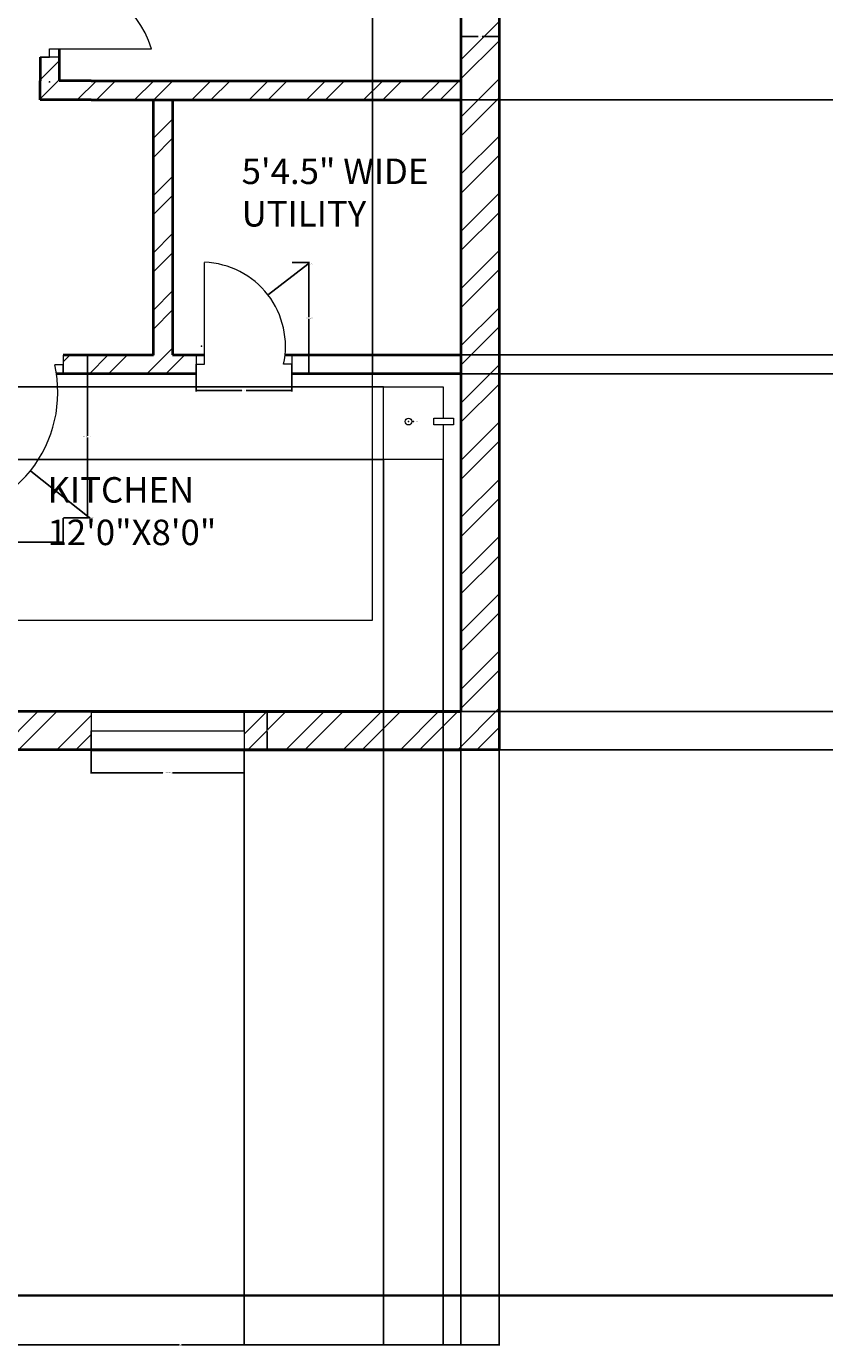
# Model space of a CAD drawing. Units: inches. Extents: x 1355 to 2746, y 1171 to 2751.
# Tile 3 of 24: x 1830 to 2017, y 1171 to 1482. Entities that reach past the tile are written whole.
import ezdxf

# ---------------------------------------------------------------- set-up
doc = ezdxf.new("R2010")
doc.units = ezdxf.units.IN
for name, color, linetype, lineweight in [('A-ANNO-DIMS', 2, 'Continuous', 18), ('A-ANNO-TTLB', 7, 'Continuous', 35), ('A-AREA-IDEN', 7, 'Continuous', 18), ('A-DOOR', 3, 'Continuous', 20), ('A-FLOR-CASE', 30, 'Continuous', 20), ('A-FLOR-FIXT', 9, 'Continuous', 18), ('A-GLAZ', 4, 'Continuous', 18), ('A-WALL', 7, 'Continuous', 40), ('A-WALL-PATT', 252, 'Continuous', 13)]:
    doc.layers.add(name, color=color, linetype=linetype, lineweight=lineweight)
doc.styles.get("Standard").update_dxf_attribs({"font": 'arial.ttf'})
doc.dimstyles.get("Standard").update_dxf_attribs({"dimtxt": 0.18, "dimasz": 0.18, "dimexe": 0.18, "dimexo": 0.0625, "dimgap": 0.09, "dimtad": 0, "dimtih": 1, "dimtoh": 1, "dimdec": 4, "dimzin": 0, "dimdsep": 46, "dimtxsty": 'Standard', "dimcen": 0.09, "dimadec": 0, "dimazin": 0, "dimtfac": 1, "dimtdec": 4, "dimtofl": 0, "dimtmove": 0, "dimatfit": 3, "dimfxl": 1, "dimtolj": 1, "dimtzin": 0, "dimarcsym": 0})

# ---------------------------------------------------------------- blocks, each defined once
blk = doc.blocks.new('WINDOW-PLAN-36')
for p, q in [((0, 9), (0, 0)), ((36, 4.5), (36, 9)), ((36, 9), (36, 0)), ((0, 0), (0, 4.5)), ((0, 4.5), (36, 4.5))]:
    blk.add_line(p, q)
blk = doc.blocks.new('DOOR-WC-SE')
for p, q in [((0, 21.41), (4.5, 21.41)), ((4.5, 21.41), (2.25, 21.41)), ((2.25, 21.41), (2.25, 19.41)), ((2.25, 0), (2.25, 2)), ((2.25, 2), (26.25, 2)), ((4.5, 0), (0, 0)), ((0, 0), (2.25, 0))]:
    blk.add_line(p, q)
blk.add_arc((2.25, -5.83), 25.25, 18.0786, 90)
blk = doc.blocks.new('DOOR-UTILITY-S')
for p, q in [((2, 2.25), (2, 26.25)), ((0, 4.5), (0, 0)), ((22.55, 4.5), (22.55, 0)), ((0, 0), (0, 2.25)), ((0, 2.25), (2, 2.25)), ((22.55, 2.25), (20.55, 2.25)), ((22.55, 0), (22.55, 2.25))]:
    blk.add_line(p, q)
blk.add_arc((1.26, 6.51), 19.76, 347.5613, 87.8563)
blk = doc.blocks.new('DOOR-KITCHEN-S')
for p, q in [((0, 38.25), (0, 33.75)), ((32.75, 38.25), (32.75, 33.89)), ((0, 33.75), (0, 36)), ((0, 36), (2, 36)), ((2, 36), (2, 0)), ((32.75, 36), (30.75, 36)), ((32.75, 33.89), (32.75, 36))]:
    blk.add_line(p, q)
blk.add_arc((2, 29.48), 29.48, 270, 12.7851)
blk = doc.blocks.new('*D43')
at = {"layer": 'A-ANNO-DIMS', "color": 0, "lineweight": -2, "transparency": 16777216}
for p, q in [((1844.71, 1311.24), (1844.71, 1305.72)), ((1880.71, 1311.24), (1880.71, 1305.72)), ((1844.89, 1305.9), (1861.59, 1305.9)), ((1880.53, 1305.9), (1863.83, 1305.9))]:
    blk.add_line(p, q, dxfattribs=at)
at = {"layer": 'A-ANNO-DIMS', "color": 0, "transparency": 16777216}
for points in [[(1844.89, 1305.93), (1844.89, 1305.87), (1844.71, 1305.9)], [(1880.53, 1305.93), (1880.53, 1305.87), (1880.71, 1305.9)]]:
    blk.add_solid(points, dxfattribs=at)
at = {"layer": 'Defpoints', "color": 0, "transparency": 16777216}
for p in [(1844.71, 1311.3), (1880.71, 1311.3), (1880.71, 1305.9)]:
    blk.add_point(p, dxfattribs=at)
at = {"layer": 'A-ANNO-DIMS', "color": 0, "transparency": 16777216, "insert": (1862.71, 1305.9), "char_height": 0.18, "attachment_point": 5}
blk.add_mtext('\\A1;WINDOW 36 TYP.', dxfattribs=at)
blk = doc.blocks.new('*D44')
at = {"layer": 'A-ANNO-DIMS', "color": 0, "lineweight": -2, "transparency": 16777216}
for p, q in [((1880.77, 1320.3), (1886.29, 1320.3)), ((1886.11, 1320.12), (1886.11, 1315.98)), ((1886.11, 1311.48), (1886.11, 1315.62)), ((1880.77, 1311.3), (1886.29, 1311.3))]:
    blk.add_line(p, q, dxfattribs=at)
at = {"layer": 'A-ANNO-DIMS', "color": 0, "transparency": 16777216}
for points in [[(1886.08, 1320.12), (1886.14, 1320.12), (1886.11, 1320.3)], [(1886.08, 1311.48), (1886.14, 1311.48), (1886.11, 1311.3)]]:
    blk.add_solid(points, dxfattribs=at)
at = {"layer": 'Defpoints', "color": 0, "transparency": 16777216}
for p in [(1880.71, 1320.3), (1886.11, 1320.3), (1880.71, 1311.3)]:
    blk.add_point(p, dxfattribs=at)
at = {"layer": 'A-ANNO-DIMS', "color": 0, "transparency": 16777216, "insert": (1886.11, 1315.8), "char_height": 0.18, "attachment_point": 5}
blk.add_mtext('\\A1;9 TYP.', dxfattribs=at)
blk = doc.blocks.new('*D52')
at = {"layer": 'A-ANNO-DIMS', "color": 0, "lineweight": -2, "transparency": 16777216}
for p, q in [((1931.71, 1482.72), (1931.71, 1479)), ((1940.71, 1482.72), (1940.71, 1479)), ((1931.89, 1479.18), (1935.75, 1479.18)), ((1940.53, 1479.18), (1936.67, 1479.18))]:
    blk.add_line(p, q, dxfattribs=at)
at = {"layer": 'A-ANNO-DIMS', "color": 0, "transparency": 16777216}
for points in [[(1931.89, 1479.21), (1931.89, 1479.15), (1931.71, 1479.18)], [(1940.53, 1479.21), (1940.53, 1479.15), (1940.71, 1479.18)]]:
    blk.add_solid(points, dxfattribs=at)
at = {"layer": 'Defpoints', "color": 0, "transparency": 16777216}
for p in [(1931.71, 1482.78), (1940.71, 1482.78), (1940.71, 1479.18)]:
    blk.add_point(p, dxfattribs=at)
at = {"layer": 'A-ANNO-DIMS', "color": 0, "transparency": 16777216, "insert": (1936.21, 1479.18), "char_height": 0.18, "attachment_point": 5}
blk.add_mtext('\\A1;9 TYP.', dxfattribs=at)
blk = doc.blocks.new('*D71')
at = {"layer": 'A-ANNO-DIMS', "color": 0, "lineweight": -2, "transparency": 16777216}
for p, q in [((1892.04, 1426.05), (1896.09, 1426.05)), ((1895.91, 1425.87), (1895.91, 1413.11)), ((1895.91, 1399.98), (1895.91, 1412.74)), ((1892.04, 1399.8), (1896.09, 1399.8))]:
    blk.add_line(p, q, dxfattribs=at)
at = {"layer": 'A-ANNO-DIMS', "color": 0, "transparency": 16777216}
for points in [[(1895.88, 1425.87), (1895.94, 1425.87), (1895.91, 1426.05)], [(1895.88, 1399.98), (1895.94, 1399.98), (1895.91, 1399.8)]]:
    blk.add_solid(points, dxfattribs=at)
at = {"layer": 'Defpoints', "color": 0, "transparency": 16777216}
for p in [(1891.97, 1426.05), (1895.91, 1426.05), (1891.97, 1399.8)]:
    blk.add_point(p, dxfattribs=at)
at = {"layer": 'A-ANNO-DIMS', "color": 0, "transparency": 16777216, "insert": (1895.91, 1412.93), "char_height": 0.18, "attachment_point": 5}
blk.add_mtext('\\A1;UTIL DOOR 26 TYP.', dxfattribs=at)
blk = doc.blocks.new('*D72')
at = {"layer": 'A-ANNO-DIMS', "color": 0, "lineweight": -2, "transparency": 16777216}
for p, q in [((1869.42, 1399.74), (1869.42, 1395.68)), ((1891.97, 1399.74), (1891.97, 1395.68)), ((1869.6, 1395.86), (1880.17, 1395.86)), ((1891.79, 1395.86), (1881.23, 1395.86))]:
    blk.add_line(p, q, dxfattribs=at)
at = {"layer": 'A-ANNO-DIMS', "color": 0, "transparency": 16777216}
for points in [[(1869.6, 1395.89), (1869.6, 1395.83), (1869.42, 1395.86)], [(1891.79, 1395.89), (1891.79, 1395.83), (1891.97, 1395.86)]]:
    blk.add_solid(points, dxfattribs=at)
at = {"layer": 'Defpoints', "color": 0, "transparency": 16777216}
for p in [(1869.42, 1399.8), (1891.97, 1399.8), (1891.97, 1395.86)]:
    blk.add_point(p, dxfattribs=at)
at = {"layer": 'A-ANNO-DIMS', "color": 0, "transparency": 16777216, "insert": (1880.7, 1395.86), "char_height": 0.18, "attachment_point": 5}
blk.add_mtext('\\A1;23 TYP.', dxfattribs=at)
blk = doc.blocks.new('*D73')
at = {"layer": 'A-ANNO-DIMS', "color": 0, "lineweight": -2, "transparency": 16777216}
for p, q in [((1838.22, 1404.17), (1844.07, 1404.17)), ((1843.89, 1403.99), (1843.89, 1385.22)), ((1843.89, 1366.1), (1843.89, 1384.86)), ((1838.22, 1365.92), (1844.07, 1365.92))]:
    blk.add_line(p, q, dxfattribs=at)
at = {"layer": 'A-ANNO-DIMS', "color": 0, "transparency": 16777216}
for points in [[(1843.86, 1403.99), (1843.92, 1403.99), (1843.89, 1404.17)], [(1843.86, 1366.1), (1843.92, 1366.1), (1843.89, 1365.92)]]:
    blk.add_solid(points, dxfattribs=at)
at = {"layer": 'Defpoints', "color": 0, "transparency": 16777216}
for p in [(1838.15, 1404.17), (1843.89, 1404.17), (1838.15, 1365.92)]:
    blk.add_point(p, dxfattribs=at)
at = {"layer": 'A-ANNO-DIMS', "color": 0, "transparency": 16777216, "insert": (1843.89, 1385.04), "char_height": 0.18, "attachment_point": 5}
blk.add_mtext('\\A1;KIT DOOR 38 TYP.', dxfattribs=at)
blk = doc.blocks.new('*D74')
at = {"layer": 'A-ANNO-DIMS', "color": 0, "lineweight": -2, "transparency": 16777216}
for p, q in [((1805.41, 1365.85), (1805.41, 1360)), ((1838.15, 1365.85), (1838.15, 1360)), ((1805.59, 1360.18), (1821.25, 1360.18)), ((1837.97, 1360.18), (1822.31, 1360.18))]:
    blk.add_line(p, q, dxfattribs=at)
at = {"layer": 'A-ANNO-DIMS', "color": 0, "transparency": 16777216}
for points in [[(1805.59, 1360.21), (1805.59, 1360.15), (1805.41, 1360.18)], [(1837.97, 1360.21), (1837.97, 1360.15), (1838.15, 1360.18)]]:
    blk.add_solid(points, dxfattribs=at)
at = {"layer": 'Defpoints', "color": 0, "transparency": 16777216}
for p in [(1805.41, 1365.92), (1838.15, 1365.92), (1838.15, 1360.18)]:
    blk.add_point(p, dxfattribs=at)
at = {"layer": 'A-ANNO-DIMS', "color": 0, "transparency": 16777216, "insert": (1821.78, 1360.18), "char_height": 0.18, "attachment_point": 5}
blk.add_mtext('\\A1;33 TYP.', dxfattribs=at)
blk = doc.blocks.new('*D106')
at = {"layer": 'A-ANNO-DIMS', "color": 0, "lineweight": -2, "transparency": 16777216}
for p, q in [((2031.09, 1557.85), (1407.53, 1557.85)), ((1407.71, 1557.67), (1407.71, 1434.76)), ((1407.71, 1311.48), (1407.71, 1434.39)), ((2080.33, 1311.3), (1407.53, 1311.3))]:
    blk.add_line(p, q, dxfattribs=at)
at = {"layer": 'A-ANNO-DIMS', "color": 0, "transparency": 16777216}
for points in [[(1407.68, 1557.67), (1407.74, 1557.67), (1407.71, 1557.85)], [(1407.68, 1311.48), (1407.74, 1311.48), (1407.71, 1311.3)]]:
    blk.add_solid(points, dxfattribs=at)
at = {"layer": 'Defpoints', "color": 0, "transparency": 16777216}
for p in [(1407.71, 1557.85), (2031.15, 1557.85), (2080.39, 1311.3)]:
    blk.add_point(p, dxfattribs=at)
at = {"layer": 'A-ANNO-DIMS', "color": 0, "transparency": 16777216, "insert": (1407.71, 1434.57), "char_height": 0.18, "attachment_point": 5}
blk.add_mtext('\\A1;246.54', dxfattribs=at)
blk = doc.blocks.new('*D141')
at = {"layer": 'A-ANNO-DIMS', "color": 0, "lineweight": -2, "transparency": 16777216}
for p, q in [((1799.71, 1320.24), (1799.71, 1171.06)), ((1931.71, 1320.24), (1931.71, 1171.06)), ((1799.89, 1171.24), (1865.43, 1171.24)), ((1931.53, 1171.24), (1865.99, 1171.24))]:
    blk.add_line(p, q, dxfattribs=at)
at = {"layer": 'A-ANNO-DIMS', "color": 0, "transparency": 16777216}
for points in [[(1799.89, 1171.27), (1799.89, 1171.21), (1799.71, 1171.24)], [(1931.53, 1171.27), (1931.53, 1171.21), (1931.71, 1171.24)]]:
    blk.add_solid(points, dxfattribs=at)
at = {"layer": 'Defpoints', "color": 0, "transparency": 16777216}
for p in [(1799.71, 1320.3), (1931.71, 1320.3), (1931.71, 1171.24)]:
    blk.add_point(p, dxfattribs=at)
at = {"layer": 'A-ANNO-DIMS', "color": 0, "transparency": 16777216, "insert": (1865.71, 1171.24), "char_height": 0.18, "attachment_point": 5}
blk.add_mtext('\\A1;132', dxfattribs=at)
blk = doc.blocks.new('*D142')
at = {"layer": 'A-ANNO-DIMS', "color": 0, "lineweight": -2, "transparency": 16777216}
for p, q in [((1931.77, 1399.8), (2648.07, 1399.8)), ((2647.89, 1399.62), (2647.89, 1360.23)), ((2647.89, 1320.48), (2647.89, 1359.87)), ((1931.77, 1320.3), (2648.07, 1320.3))]:
    blk.add_line(p, q, dxfattribs=at)
at = {"layer": 'A-ANNO-DIMS', "color": 0, "transparency": 16777216}
for points in [[(2647.86, 1399.62), (2647.92, 1399.62), (2647.89, 1399.8)], [(2647.86, 1320.48), (2647.92, 1320.48), (2647.89, 1320.3)]]:
    blk.add_solid(points, dxfattribs=at)
at = {"layer": 'Defpoints', "color": 0, "transparency": 16777216}
for p in [(1931.71, 1399.8), (2647.89, 1399.8), (1931.71, 1320.3)]:
    blk.add_point(p, dxfattribs=at)
at = {"layer": 'A-ANNO-DIMS', "color": 0, "transparency": 16777216, "insert": (2647.89, 1360.05), "char_height": 0.18, "attachment_point": 5}
blk.add_mtext('\\A1;79.5', dxfattribs=at)
blk = doc.blocks.new('*D143')
at = {"layer": 'A-ANNO-DIMS', "color": 0, "lineweight": -2, "transparency": 16777216}
for p, q in [((1931.77, 1464.3), (2648.07, 1464.3)), ((2647.89, 1464.12), (2647.89, 1434.48)), ((2647.89, 1404.48), (2647.89, 1434.12)), ((1931.77, 1404.3), (2648.07, 1404.3))]:
    blk.add_line(p, q, dxfattribs=at)
at = {"layer": 'A-ANNO-DIMS', "color": 0, "transparency": 16777216}
for points in [[(2647.86, 1464.12), (2647.92, 1464.12), (2647.89, 1464.3)], [(2647.86, 1404.48), (2647.92, 1404.48), (2647.89, 1404.3)]]:
    blk.add_solid(points, dxfattribs=at)
at = {"layer": 'Defpoints', "color": 0, "transparency": 16777216}
for p in [(1931.71, 1464.3), (2647.89, 1464.3), (1931.71, 1404.3)]:
    blk.add_point(p, dxfattribs=at)
at = {"layer": 'A-ANNO-DIMS', "color": 0, "transparency": 16777216, "insert": (2647.89, 1434.3), "char_height": 0.18, "attachment_point": 5}
blk.add_mtext('\\A1;60', dxfattribs=at)
blk = doc.blocks.new('*D144')
at = {"layer": 'A-ANNO-DIMS', "color": 0, "lineweight": -2, "transparency": 16777216}
for p, q in [((1880.71, 1311.24), (1880.71, 1171.06)), ((1940.71, 1311.24), (1940.71, 1171.06)), ((1880.89, 1171.24), (1910.49, 1171.24)), ((1940.53, 1171.24), (1910.93, 1171.24))]:
    blk.add_line(p, q, dxfattribs=at)
at = {"layer": 'A-ANNO-DIMS', "color": 0, "transparency": 16777216}
for points in [[(1880.89, 1171.27), (1880.89, 1171.21), (1880.71, 1171.24)], [(1940.53, 1171.27), (1940.53, 1171.21), (1940.71, 1171.24)]]:
    blk.add_solid(points, dxfattribs=at)
at = {"layer": 'Defpoints', "color": 0, "transparency": 16777216}
for p in [(1880.71, 1311.3), (1940.71, 1311.3), (1940.71, 1171.24)]:
    blk.add_point(p, dxfattribs=at)
at = {"layer": 'A-ANNO-DIMS', "color": 0, "transparency": 16777216, "insert": (1910.71, 1171.24), "char_height": 0.18, "attachment_point": 5}
blk.add_mtext('\\A1;60', dxfattribs=at)
blk = doc.blocks.new('*D145')
at = {"layer": 'A-ANNO-DIMS', "color": 0, "lineweight": -2, "transparency": 16777216}
for p, q in [((1910.88, 1399.86), (1910.88, 2716.58)), ((1911.06, 2716.4), (1920.83, 2716.4)), ((1931.53, 2716.4), (1921.76, 2716.4)), ((1931.71, 1399.86), (1931.71, 2716.58))]:
    blk.add_line(p, q, dxfattribs=at)
at = {"layer": 'A-ANNO-DIMS', "color": 0, "transparency": 16777216}
for points in [[(1911.06, 2716.43), (1911.06, 2716.37), (1910.88, 2716.4)], [(1931.53, 2716.43), (1931.53, 2716.37), (1931.71, 2716.4)]]:
    blk.add_solid(points, dxfattribs=at)
at = {"layer": 'Defpoints', "color": 0, "transparency": 16777216}
for p in [(1931.71, 2716.4), (1910.88, 1399.8), (1931.71, 1399.8)]:
    blk.add_point(p, dxfattribs=at)
at = {"layer": 'A-ANNO-DIMS', "color": 0, "transparency": 16777216, "insert": (1921.3, 2716.4), "char_height": 0.18, "attachment_point": 5}
blk.add_mtext('\\A1;20.824', dxfattribs=at)
blk = doc.blocks.new('*D146')
at = {"layer": 'A-ANNO-DIMS', "color": 0, "lineweight": -2, "transparency": 16777216}
for p, q in [((1913.53, 1379.56), (1913.53, 1171.06)), ((1927.55, 1379.56), (1927.55, 1171.06)), ((1913.71, 1171.24), (1920.08, 1171.24)), ((1927.37, 1171.24), (1920.99, 1171.24))]:
    blk.add_line(p, q, dxfattribs=at)
at = {"layer": 'A-ANNO-DIMS', "color": 0, "transparency": 16777216}
for points in [[(1913.71, 1171.27), (1913.71, 1171.21), (1913.53, 1171.24)], [(1927.37, 1171.27), (1927.37, 1171.21), (1927.55, 1171.24)]]:
    blk.add_solid(points, dxfattribs=at)
at = {"layer": 'Defpoints', "color": 0, "transparency": 16777216}
for p in [(1913.53, 1379.62), (1927.55, 1379.62), (1927.55, 1171.24)]:
    blk.add_point(p, dxfattribs=at)
at = {"layer": 'A-ANNO-DIMS', "color": 0, "transparency": 16777216, "insert": (1920.54, 1171.24), "char_height": 0.18, "attachment_point": 5}
blk.add_mtext('\\A1;14.014', dxfattribs=at)
blk = doc.blocks.new('*D147')
at = {"layer": 'A-ANNO-DIMS', "color": 0, "lineweight": -2, "transparency": 16777216}
for p, q in [((1913.47, 1396.75), (1407.53, 1396.75)), ((1407.71, 1396.57), (1407.71, 1388.37)), ((1407.71, 1379.8), (1407.71, 1388.01)), ((1913.47, 1379.62), (1407.53, 1379.62))]:
    blk.add_line(p, q, dxfattribs=at)
at = {"layer": 'A-ANNO-DIMS', "color": 0, "transparency": 16777216}
for points in [[(1407.68, 1396.57), (1407.74, 1396.57), (1407.71, 1396.75)], [(1407.68, 1379.8), (1407.74, 1379.8), (1407.71, 1379.62)]]:
    blk.add_solid(points, dxfattribs=at)
at = {"layer": 'Defpoints', "color": 0, "transparency": 16777216}
for p in [(1407.71, 1396.75), (1913.53, 1396.75), (1913.53, 1379.62)]:
    blk.add_point(p, dxfattribs=at)
at = {"layer": 'A-ANNO-DIMS', "color": 0, "transparency": 16777216, "insert": (1407.71, 1388.19), "char_height": 0.18, "attachment_point": 5}
blk.add_mtext('\\A1;17.13', dxfattribs=at)
blk = doc.blocks.new('*D149')
at = {"layer": 'A-ANNO-DIMS', "color": 0, "lineweight": -2, "transparency": 16777216}
for p, q in [((1919.3, 1388.57), (1919.48, 1388.57)), ((1919.39, 1388.48), (1919.39, 1388.66)), ((1920.65, 1388.57), (1920.36, 1388.57))]:
    blk.add_line(p, q, dxfattribs=at)
at = {"layer": 'A-ANNO-DIMS', "color": 0, "transparency": 16777216}
blk.add_solid([(1920.36, 1388.6), (1920.36, 1388.54), (1920.18, 1388.57)], dxfattribs=at)
at = {"layer": 'Defpoints', "color": 0, "transparency": 16777216}
for p in [(1918.6, 1388.56), (1920.18, 1388.57)]:
    blk.add_point(p, dxfattribs=at)
at = {"layer": 'A-ANNO-DIMS', "color": 0, "transparency": 16777216, "insert": (1921.08, 1388.57), "char_height": 0.18, "attachment_point": 5}
blk.add_mtext('\\A1;∅1.58', dxfattribs=at)
blk = doc.blocks.new('*D151')
at = {"layer": 'A-ANNO-DIMS', "color": 0, "lineweight": -2, "transparency": 16777216}
for p, q in [((1807.32, 1395.39), (1807.5, 1395.39)), ((1807.41, 1395.3), (1807.41, 1395.48)), ((1844.26, 1365.96), (1830.58, 1376.89)), ((1844.44, 1365.96), (1844.26, 1365.96))]:
    blk.add_line(p, q, dxfattribs=at)
at = {"layer": 'A-ANNO-DIMS', "color": 0, "transparency": 16777216}
blk.add_solid([(1830.6, 1376.91), (1830.56, 1376.86), (1830.44, 1377)], dxfattribs=at)
at = {"layer": 'Defpoints', "color": 0, "transparency": 16777216}
for p in [(1807.41, 1395.39), (1830.44, 1377)]:
    blk.add_point(p, dxfattribs=at)
at = {"layer": 'A-ANNO-DIMS', "color": 0, "transparency": 16777216, "insert": (1844.99, 1365.96), "char_height": 0.18, "attachment_point": 5}
blk.add_mtext('\\A1;R29.477', dxfattribs=at)
blk = doc.blocks.new('*D161')
at = {"layer": 'A-ANNO-DIMS', "color": 0, "lineweight": -2, "transparency": 16777216}
for p, q in [((1858.68, 1501.2), (1849.89, 1489.09)), ((1858.86, 1501.2), (1858.68, 1501.2)), ((1834.87, 1468.51), (1835.05, 1468.51)), ((1834.96, 1468.42), (1834.96, 1468.6))]:
    blk.add_line(p, q, dxfattribs=at)
at = {"layer": 'A-ANNO-DIMS', "color": 0, "transparency": 16777216}
blk.add_solid([(1849.87, 1489.1), (1849.91, 1489.07), (1849.78, 1488.94)], dxfattribs=at)
at = {"layer": 'Defpoints', "color": 0, "transparency": 16777216}
for p in [(1849.78, 1488.94), (1834.96, 1468.51)]:
    blk.add_point(p, dxfattribs=at)
at = {"layer": 'A-ANNO-DIMS', "color": 0, "transparency": 16777216, "insert": (1859.41, 1501.2), "char_height": 0.18, "attachment_point": 5}
blk.add_mtext('\\A1;R25.246', dxfattribs=at)
blk = doc.blocks.new('*D163')
at = {"layer": 'A-ANNO-DIMS', "color": 0, "lineweight": -2, "transparency": 16777216}
for p, q in [((1895.69, 1425.64), (1886.45, 1418.5)), ((1895.87, 1425.64), (1895.69, 1425.64)), ((1870.59, 1406.31), (1870.77, 1406.31)), ((1870.68, 1406.22), (1870.68, 1406.4))]:
    blk.add_line(p, q, dxfattribs=at)
at = {"layer": 'A-ANNO-DIMS', "color": 0, "transparency": 16777216}
blk.add_solid([(1886.43, 1418.53), (1886.47, 1418.48), (1886.31, 1418.39)], dxfattribs=at)
at = {"layer": 'Defpoints', "color": 0, "transparency": 16777216}
for p in [(1886.31, 1418.39), (1870.68, 1406.31)]:
    blk.add_point(p, dxfattribs=at)
at = {"layer": 'A-ANNO-DIMS', "color": 0, "transparency": 16777216, "insert": (1896.35, 1425.64), "char_height": 0.18, "attachment_point": 5}
blk.add_mtext('\\A1;R19.76', dxfattribs=at)

msp = doc.modelspace()

# ---------------------------------------------------------------- hatches: boundary and pattern name
at = {"layer": 'A-WALL-PATT'}
h = msp.add_hatch(dxfattribs=at)
h.set_pattern_fill('ANSI32', color=256)
h.paths.add_polyline_path([(1660.2083, 2139.3018), (1614.5977, 2139.3018), (1614.5977, 2130.3018), (1655.7083, 2130.3018), (1655.7083, 1981.8018), (1660.2083, 1981.8018), (1660.2083, 2090.7225), (1692.5832, 2090.7225), (1692.5832, 2095.2225), (1660.2083, 2095.2225)])
h.paths.add_polyline_path([(1523.7083, 2130.3018), (1554.5977, 2130.3018), (1554.5977, 2134.8018), (1554.5977, 2139.3018), (1514.7083, 2139.3018), (1514.7083, 2071.8385), (1523.7083, 2071.8385)])
h.paths.add_polyline_path([(1940.7083, 2139.3018), (1883.7928, 2139.3018), (1883.7928, 2130.3018), (1931.7083, 2130.3018), (1931.7083, 2098.3333), (1940.7083, 2098.3333)])
h.paths.add_polyline_path([(1799.7083, 2130.3018), (1823.7928, 2130.3018), (1823.7928, 2134.8018), (1823.7928, 2139.3018), (1795.2083, 2139.3018), (1795.2083, 2130.3018), (1795.2083, 2095.2225), (1759.2134, 2095.2225), (1759.2134, 2090.7225), (1795.2083, 2090.7225), (1795.2083, 1981.8018), (1799.7083, 1981.8018), (1799.7083, 1986.3018)])
h.paths.add_polyline_path([(1940.7083, 2038.3333), (1931.7083, 2038.3333), (1931.7083, 1986.3018), (1832.7083, 1986.3018), (1832.7083, 1947.1338), (1837.2083, 1947.1338), (1837.2083, 1981.8018), (1931.7083, 1981.8018), (1931.7083, 1967.1939), (1940.7083, 1967.1939)])
h.paths.add_polyline_path([(1940.7083, 1943.1939), (1931.7083, 1943.1939), (1931.7083, 1921.8018), (1837.2083, 1921.8018), (1837.2083, 1926.0511), (1832.7083, 1926.0511), (1832.7083, 1917.3018), (1931.7083, 1917.3018), (1931.7083, 1908.3321), (1940.7083, 1908.3321)])
h.paths.add_polyline_path([(1940.7083, 1884.3321), (1931.7083, 1884.3321), (1931.7083, 1869.3018), (1899.4583, 1869.3018), (1899.4583, 1864.8018), (1931.7083, 1864.8018), (1931.7083, 1773.3018), (1786.5143, 1773.3018), (1786.5143, 1764.3018), (1844.7083, 1764.3018), (1844.7083, 1748.9343), (1853.7083, 1748.9343), (1853.7083, 1764.3018), (1931.7083, 1764.3018), (1931.7083, 1652.9424), (1940.7083, 1652.9424)])
h.paths.add_polyline_path([(1799.7083, 1864.8018), (1806.0522, 1864.8018), (1806.0522, 1867.0518), (1806.0522, 1869.3018), (1799.7083, 1869.3018), (1799.7083, 1917.3018), (1799.7083, 1921.8018), (1795.2083, 1921.8018), (1795.2083, 1773.3018), (1799.7083, 1773.3018)])
h.paths.add_polyline_path([(1872.8988, 1867.0518), (1872.8988, 1869.3018), (1867.2083, 1869.3018), (1867.2083, 1917.3018), (1862.7083, 1917.3018), (1862.7083, 1869.3018), (1836.9546, 1869.3018), (1836.9546, 1864.8018), (1862.7083, 1864.8018), (1872.8988, 1864.8018)])
h.paths.add_polyline_path([(1749.2197, 1773.3018), (1655.7083, 1773.3018), (1523.7083, 1773.3018), (1523.7083, 1828.4963), (1514.7083, 1828.4963), (1514.7083, 1753.9033), (1519.2083, 1753.9033), (1523.7083, 1753.9033), (1523.7083, 1764.3018), (1655.7083, 1764.3018), (1749.2197, 1764.3018), (1749.2197, 1768.8018)])
h.paths.add_polyline_path([(1660.2083, 1921.8018), (1655.7083, 1921.8018), (1655.7083, 1917.3018), (1655.7083, 1773.3018), (1660.2083, 1773.3018)])
h.paths.add_polyline_path([(1523.7083, 2011.8385), (1514.7083, 2011.8385), (1514.7083, 1973.114), (1519.2083, 1973.114), (1523.7083, 1973.114), (1523.7083, 1976.8227), (1523.7083, 1981.8018), (1618.2083, 1981.8018), (1618.2083, 1921.8018), (1553.707, 1921.8018), (1553.707, 1917.3018), (1622.7083, 1917.3018), (1622.7083, 1919.5518), (1622.7083, 1921.8018), (1622.7083, 1986.3018), (1523.7083, 1986.3018)])
h.paths.add_polyline_path([(1529.6686, 1919.5518), (1529.6686, 1921.8018), (1523.7083, 1921.8018), (1523.7083, 1949.114), (1514.7083, 1949.114), (1514.7083, 1888.4963), (1523.7083, 1888.4963), (1523.7083, 1917.3018), (1529.6686, 1917.3018)])
h.paths.add_polyline_path([(1538.9419, 1775.643), (1585.5504, 1775.643), (1585.5504, 1798.0318), (1538.9419, 1798.0318)], flags=25)
h.paths.add_polyline_path([(1696.7097, 1497.3356), (1769.5651, 1497.3356), (1769.5651, 1523.4559), (1696.7097, 1523.4559)], flags=9)
h.paths.add_polyline_path([(1629.1643, 1230.5133), (1877.0879, 1230.5133), (1877.0879, 1267.606), (1629.1643, 1267.606)], flags=9)
h.paths.add_polyline_path([(2533.4462, 2215.4033), (2579.9292, 2215.4033), (2579.9292, 2231.889), (2533.4462, 2231.889)], flags=9)
h.paths.add_polyline_path([(2540.822, 2515.6945), (2594.2245, 2515.6945), (2594.2245, 2545.5463), (2540.822, 2545.5463)], flags=9)
h.paths.add_polyline_path([(2535.9857, 2588.2819), (2582.4687, 2588.2819), (2582.4687, 2604.7675), (2535.9857, 2604.7675)], flags=9)
h.paths.add_polyline_path([(2537.1627, 2617.1172), (2649.1245, 2617.1172), (2649.1245, 2633.6029), (2537.1627, 2633.6029)], flags=9)
h.paths.add_polyline_path([(2218.0051, 2168.228), (2363.9573, 2168.228), (2363.9573, 2205.3208), (2218.0051, 2205.3208)], flags=9)
h.paths.add_polyline_path([(1650.2156, 2165.3631), (1800.3547, 2165.3631), (1800.3547, 2202.4559), (1650.2156, 2202.4559)], flags=9)
h.paths.add_polyline_path([(2553.9592, 1610.7663), (2588.4203, 1610.7663), (2588.4203, 1660.2233), (2553.9592, 1660.2233)], flags=9)
h.paths.add_polyline_path([(1549.0868, 1648.2033), (1595.6952, 1648.2033), (1595.6952, 1670.5921), (1549.0868, 1670.5921)], flags=9)
h.paths.add_polyline_path([(1546.9525, 1502.0931), (1583.3413, 1502.0931), (1583.3413, 1524.4819), (1546.9525, 1524.4819)], flags=9)
h.paths.add_polyline_path([(1540.7704, 1433.4431), (1587.3788, 1433.4431), (1587.3788, 1455.8319), (1540.7704, 1455.8319)], flags=9)
h.paths.add_polyline_path([(1683.6524, 1321.5269), (1760.6169, 1321.5269), (1760.6169, 1333.8911), (1683.6524, 1333.8911)], flags=9)
h.paths.add_polyline_path([(1832.0485, 1356.0874), (1873.0989, 1356.0874), (1873.0989, 1378.4762), (1832.0485, 1378.4762)], flags=9)
h.paths.add_polyline_path([(1877.9694, 1431.2138), (1926.3827, 1431.2138), (1926.3827, 1453.578), (1877.9694, 1453.578)], flags=9)
h.paths.add_polyline_path([(1847.3106, 1499.8371), (1883.6994, 1499.8371), (1883.6994, 1522.2259), (1847.3106, 1522.2259)], flags=9)
h.paths.add_polyline_path([(1813.7015, 1640.7287), (1860.3099, 1640.7287), (1860.3099, 1663.1175), (1813.7015, 1663.1175)], flags=9)
h.paths.add_polyline_path([(1876.2576, 1710.2471), (1912.9452, 1710.2471), (1912.9452, 1732.6359), (1876.2576, 1732.6359)], flags=25)
h.paths.add_polyline_path([(1695.9163, 1715.3064), (1736.9668, 1715.3064), (1736.9668, 1737.6952), (1695.9163, 1737.6952)], flags=9)
h.paths.add_polyline_path([(1881.8583, 1888.9094), (1930.2717, 1888.9094), (1930.2717, 1911.2737), (1881.8583, 1911.2737)], flags=9)
h.paths.add_polyline_path([(1823.9298, 1798.6431), (1864.9803, 1798.6431), (1864.9803, 1821.0319), (1823.9298, 1821.0319)], flags=25)
h.paths.add_polyline_path([(1845.6062, 1948.1408), (1881.995, 1948.1408), (1881.995, 1970.5296), (1845.6062, 1970.5296)], flags=25)
h.paths.add_polyline_path([(1849.027, 1991.5151), (1895.6355, 1991.5151), (1895.6355, 2013.9039), (1849.027, 2013.9039)], flags=25)
h.paths.add_polyline_path([(1684.9725, 2113.8416), (1764.2658, 2113.8416), (1764.2658, 2126.2058), (1684.9725, 2126.2058)], flags=9)
h.paths.add_polyline_path([(1688.6193, 1913.0676), (1776.2005, 1913.0676), (1776.2005, 1935.4564), (1688.6193, 1935.4564)], flags=9)
h.paths.add_polyline_path([(1571.4689, 1930.9816), (1607.8577, 1930.9816), (1607.8577, 1953.3704), (1571.4689, 1953.3704)], flags=25)
h.paths.add_polyline_path([(1535.3581, 1998.3125), (1581.9665, 1998.3125), (1581.9665, 2020.7014), (1535.3581, 2020.7014)], flags=9)
h = msp.add_hatch(dxfattribs=at)
h.set_pattern_fill('ANSI32', color=256)
h.paths.add_polyline_path([(1749.2197, 1686.3018), (1732.6892, 1686.3018), (1523.7083, 1686.3018), (1523.7083, 1705.9033), (1514.7083, 1705.9033), (1514.7083, 1647.8732), (1519.2083, 1647.8732), (1523.7083, 1647.8732), (1523.7083, 1677.3018), (1655.7083, 1677.3018), (1655.7083, 1528.8018), (1660.2083, 1528.8018), (1660.2083, 1677.3018), (1732.6892, 1677.3018), (1749.2197, 1677.3018)])
h.paths.add_polyline_path([(1931.7083, 1686.3018), (1853.7083, 1686.3018), (1853.7083, 1703.5696), (1844.7083, 1703.5696), (1844.7083, 1686.3018), (1788.0274, 1686.3018), (1788.0274, 1677.3018), (1795.2083, 1677.3018), (1795.2083, 1528.8018), (1799.7083, 1528.8018), (1799.7083, 1677.3018), (1844.7083, 1677.3018), (1931.7083, 1677.3018)])
h.paths.add_polyline_path([(1931.7083, 1533.3018), (1844.7083, 1533.3018), (1832.7083, 1533.3018), (1832.7083, 1531.0518), (1832.7083, 1528.8018), (1832.7083, 1495.7519), (1837.2083, 1495.7519), (1837.2083, 1528.8018), (1931.7083, 1528.8018)])
h.paths.add_polyline_path([(1940.7083, 1592.9424), (1931.7083, 1592.9424), (1931.7083, 1506.7845), (1940.7083, 1506.7845)])
h.paths.add_polyline_path([(1940.7083, 1482.7845), (1936.2083, 1482.7845), (1931.7083, 1482.7845), (1931.7083, 1320.3018), (1880.7083, 1320.3018), (1880.7083, 1311.3018), (1940.7083, 1311.3018)])
h.paths.add_polyline_path([(1931.7083, 1468.8018), (1844.7083, 1468.8018), (1837.2083, 1468.8018), (1837.2083, 1474.34), (1832.7083, 1474.34), (1832.7083, 1468.8018), (1832.7083, 1464.3018), (1844.7083, 1464.3018), (1931.7083, 1464.3018)])
h.paths.add_polyline_path([(1863.8571, 1464.3018), (1859.3571, 1464.3018), (1859.3571, 1404.1662), (1838.1542, 1404.1662), (1838.1542, 1399.8018), (1869.4185, 1399.8018), (1869.4185, 1402.0518), (1869.4185, 1404.3018), (1863.8571, 1404.3018)])
h.paths.add_polyline_path([(1799.7083, 1399.6662), (1805.4082, 1399.6662), (1805.4082, 1401.9162), (1805.4082, 1404.1662), (1799.7083, 1404.1662), (1799.7083, 1464.3018), (1799.7083, 1468.8018), (1795.2083, 1468.8018), (1795.2083, 1356.2098), (1761.2597, 1356.2098), (1761.2597, 1351.7098), (1795.2083, 1351.7098), (1795.2083, 1320.3018), (1795.2083, 1311.3018), (1844.7083, 1311.3018), (1844.7083, 1315.8018), (1844.7083, 1320.3018), (1799.7083, 1320.3018)])
h.paths.add_polyline_path([(1692.9218, 1356.2098), (1660.2083, 1356.2098), (1660.2083, 1430.786), (1657.9583, 1430.786), (1655.7083, 1430.786), (1655.7083, 1320.3018), (1611.934, 1320.3018), (1611.934, 1311.3018), (1660.2083, 1311.3018), (1660.2083, 1351.7098), (1692.9218, 1351.7098)])
h.paths.add_polyline_path([(1523.7083, 1372.653), (1514.7083, 1372.653), (1514.7083, 1311.3018), (1551.934, 1311.3018), (1551.934, 1315.8018), (1551.934, 1320.3018), (1523.7083, 1320.3018)])
h.paths.add_polyline_path([(1523.7083, 1490.9023), (1514.7083, 1490.9023), (1514.7083, 1432.653), (1519.2083, 1432.653), (1523.7083, 1432.653)])
h.paths.add_polyline_path([(1660.2083, 1468.8018), (1622.7083, 1468.8018), (1622.7083, 1473.1566), (1618.2083, 1473.1566), (1618.2083, 1468.8018), (1523.7083, 1468.8018), (1523.7083, 1464.3018), (1655.7083, 1464.3018), (1655.7083, 1460.5634), (1660.2083, 1460.5634)])
h.paths.add_polyline_path([(1523.7083, 1587.8732), (1514.7083, 1587.8732), (1514.7083, 1514.9023), (1519.2083, 1514.9023), (1523.7083, 1514.9023)])
h.paths.add_polyline_path([(1622.7083, 1533.3018), (1523.7083, 1533.3018), (1523.7083, 1528.8018), (1618.2083, 1528.8018), (1618.2083, 1494.4205), (1622.7083, 1494.4205), (1622.7083, 1528.8018)])
h.paths.add_polyline_path([(1696.7097, 1497.3356), (1769.5651, 1497.3356), (1769.5651, 1523.4559), (1696.7097, 1523.4559)], flags=9)
h.paths.add_polyline_path([(1629.1643, 1230.5133), (1877.0879, 1230.5133), (1877.0879, 1267.606), (1629.1643, 1267.606)], flags=9)
h.paths.add_polyline_path([(2533.4462, 2215.4033), (2579.9292, 2215.4033), (2579.9292, 2231.889), (2533.4462, 2231.889)], flags=9)
h.paths.add_polyline_path([(2540.822, 2515.6945), (2594.2245, 2515.6945), (2594.2245, 2545.5463), (2540.822, 2545.5463)], flags=9)
h.paths.add_polyline_path([(2535.9857, 2588.2819), (2582.4687, 2588.2819), (2582.4687, 2604.7675), (2535.9857, 2604.7675)], flags=9)
h.paths.add_polyline_path([(2537.1627, 2617.1172), (2649.1245, 2617.1172), (2649.1245, 2633.6029), (2537.1627, 2633.6029)], flags=9)
h.paths.add_polyline_path([(2218.0051, 2168.228), (2363.9573, 2168.228), (2363.9573, 2205.3208), (2218.0051, 2205.3208)], flags=9)
h.paths.add_polyline_path([(1650.2156, 2165.3631), (1800.3547, 2165.3631), (1800.3547, 2202.4559), (1650.2156, 2202.4559)], flags=9)
h.paths.add_polyline_path([(2553.9592, 1610.7663), (2588.4203, 1610.7663), (2588.4203, 1660.2233), (2553.9592, 1660.2233)], flags=9)
h.paths.add_polyline_path([(1549.0868, 1648.2033), (1595.6952, 1648.2033), (1595.6952, 1670.5921), (1549.0868, 1670.5921)], flags=25)
h.paths.add_polyline_path([(1546.9525, 1502.0931), (1583.3413, 1502.0931), (1583.3413, 1524.4819), (1546.9525, 1524.4819)], flags=25)
h.paths.add_polyline_path([(1540.7704, 1433.4431), (1587.3788, 1433.4431), (1587.3788, 1455.8319), (1540.7704, 1455.8319)], flags=9)
h.paths.add_polyline_path([(1683.6524, 1321.5269), (1760.6169, 1321.5269), (1760.6169, 1333.8911), (1683.6524, 1333.8911)], flags=9)
h.paths.add_polyline_path([(1832.0485, 1356.0874), (1873.0989, 1356.0874), (1873.0989, 1378.4762), (1832.0485, 1378.4762)], flags=9)
h.paths.add_polyline_path([(1877.9694, 1431.2138), (1926.3827, 1431.2138), (1926.3827, 1453.578), (1877.9694, 1453.578)], flags=9)
h.paths.add_polyline_path([(1847.3106, 1499.8371), (1883.6994, 1499.8371), (1883.6994, 1522.2259), (1847.3106, 1522.2259)], flags=25)
h.paths.add_polyline_path([(1813.7015, 1640.7287), (1860.3099, 1640.7287), (1860.3099, 1663.1175), (1813.7015, 1663.1175)], flags=25)
h.paths.add_polyline_path([(1876.2576, 1710.2471), (1912.9452, 1710.2471), (1912.9452, 1732.6359), (1876.2576, 1732.6359)], flags=9)
h.paths.add_polyline_path([(1695.9163, 1715.3064), (1736.9668, 1715.3064), (1736.9668, 1737.6952), (1695.9163, 1737.6952)], flags=9)
h.paths.add_polyline_path([(1881.8583, 1888.9094), (1930.2717, 1888.9094), (1930.2717, 1911.2737), (1881.8583, 1911.2737)], flags=9)
h.paths.add_polyline_path([(1823.9298, 1798.6431), (1864.9803, 1798.6431), (1864.9803, 1821.0319), (1823.9298, 1821.0319)], flags=9)
h.paths.add_polyline_path([(1845.6062, 1948.1408), (1881.995, 1948.1408), (1881.995, 1970.5296), (1845.6062, 1970.5296)], flags=9)
h.paths.add_polyline_path([(1849.027, 1991.5151), (1895.6355, 1991.5151), (1895.6355, 2013.9039), (1849.027, 2013.9039)], flags=9)
h.paths.add_polyline_path([(1684.9725, 2113.8416), (1764.2658, 2113.8416), (1764.2658, 2126.2058), (1684.9725, 2126.2058)], flags=9)
h.paths.add_polyline_path([(1688.6193, 1913.0676), (1776.2005, 1913.0676), (1776.2005, 1935.4564), (1688.6193, 1935.4564)], flags=9)
h.paths.add_polyline_path([(1538.9419, 1775.643), (1585.5504, 1775.643), (1585.5504, 1798.0318), (1538.9419, 1798.0318)], flags=9)
h.paths.add_polyline_path([(1571.4689, 1930.9816), (1607.8577, 1930.9816), (1607.8577, 1953.3704), (1571.4689, 1953.3704)], flags=9)
h.paths.add_polyline_path([(1535.3581, 1998.3125), (1581.9665, 1998.3125), (1581.9665, 2020.7014), (1535.3581, 2020.7014)], flags=9)

# ---------------------------------------------------------------- linework, layer by layer
at = {"layer": 'A-ANNO-TTLB'}
msp.add_lwpolyline([(1355.0901, 2751.4741), (2746.1804, 2751.4741), (2746.1804, 1182.883), (1355.0901, 1182.883)], close=True, dxfattribs=at)
at = {"layer": 'A-FLOR-CASE'}
for p, q in [((1910.8841, 1341.7851), (1910.8841, 1399.8018)), ((1799.7083, 1341.7851), (1910.8841, 1341.7851))]:
    msp.add_line(p, q, dxfattribs=at)
at = {"layer": 'A-FLOR-FIXT'}
msp.add_lwpolyline([(1927.5454, 1387.7756), (1927.5454, 1379.6228), (1913.531, 1379.6228), (1913.531, 1396.7528), (1927.5454, 1396.7528), (1927.5454, 1389.3811)], dxfattribs=at)
msp.add_lwpolyline([(1925.3706, 1389.3811), (1929.9795, 1389.3811), (1929.9795, 1387.7756), (1925.3706, 1387.7756)], close=True, dxfattribs=at)
msp.add_circle((1919.3883, 1388.5667), 0.7911, dxfattribs=at)
at = {"layer": 'A-WALL'}
for p, q in [((1940.7083, 2139.3018), (1940.7083, 1311.3018)), ((1931.7083, 1764.3018), (1931.7083, 1320.3018)), ((1837.2083, 1476.34), (1837.2083, 1468.8018)), ((1832.7083, 1474.34), (1832.7083, 1468.8018)), ((1832.7083, 1464.3018), (1832.7083, 1468.8018)), ((1844.7083, 1468.8018), (1837.2083, 1468.8018)), ((1844.7083, 1468.8018), (1931.7083, 1468.8018)), ((1844.7083, 1464.3018), (1832.7083, 1464.3018)), ((1844.7083, 1464.3018), (1931.7083, 1464.3018)), ((1859.3571, 1404.1662), (1859.3571, 1464.3018)), ((1859.3571, 1464.3018), (1863.8571, 1464.3018)), ((1863.8571, 1464.3018), (1863.8571, 1404.3018)), ((1931.7083, 1464.3018), (1931.7083, 1399.8018)), ((1859.3571, 1404.1662), (1838.1542, 1404.1662)), ((1863.8571, 1404.3018), (1871.4185, 1404.3018)), ((1890.3354, 1404.3018), (1931.7083, 1404.3018)), ((1838.1542, 1399.8018), (1836.5535, 1399.802)), ((1869.4185, 1399.8018), (1838.1542, 1399.8018)), ((1931.7083, 1399.8018), (1891.9737, 1399.8018)), ((1931.7083, 1320.3018), (1799.7083, 1320.3018)), ((1844.7083, 1320.3018), (1931.7083, 1320.3018)), ((1940.7083, 1311.3018), (1795.2083, 1311.3018)), ((1844.7083, 1311.3018), (1931.7083, 1311.3018))]:
    msp.add_line(p, q, dxfattribs=at)

# ---------------------------------------------------------------- block references
at = {"layer": 'A-DOOR'}
for name, p in [('DOOR-WC-SE', (1832.708, 1474.34)), ('DOOR-UTILITY-S', (1869.419, 1399.802)), ('DOOR-KITCHEN-S', (1805.408, 1365.916))]:
    msp.add_blockref(name, p, dxfattribs=at)
at = {"layer": 'A-GLAZ'}
msp.add_blockref('WINDOW-PLAN-36', (1844.708, 1311.302), dxfattribs=at)

# ---------------------------------------------------------------- texts
at = {"layer": 'A-AREA-IDEN', "char_height": 6, "attachment_point": 1}
for s, width, insert in [('5\'4.5" WIDE UTILITY', 60.579997, (1880.1283, 1450.49)), ('KITCHEN\\P12\'0"X8\'0"', 140.094749, (1834.4611, 1375.4906))]:
    msp.add_mtext_dynamic_manual_height_columns(s, width=width, gutter_width=12.5, heights=[0], dxfattribs=dict(at, insert=insert))

# ---------------------------------------------------------------- dimensions: what is measured, and where the dimension line sits
at = {"layer": 'A-ANNO-DIMS'}
for base, p1, p2, override, picture, middle in [((1931.7083, 2716.3999), (1910.8841, 1399.8018), (1931.7083, 1399.8018), {"dimdec": 3, "dimlfac": 1, "dimrnd": 0, "dimzin": 0, "dimdsep": 46, "dimlunit": 2}, '*D145', (1921.2962, 2716.3999)), ((1927.5454, 1171.2388), (1913.531, 1379.6228), (1927.5454, 1379.6228), {"dimdec": 3, "dimlfac": 1, "dimrnd": 0, "dimzin": 0, "dimdsep": 46, "dimlunit": 2}, '*D146', (1920.5382, 1171.2388)), ((1931.7083, 1171.2388), (1799.7083, 1320.3018), (1931.7083, 1320.3018), {"dimdec": 0, "dimlfac": 1, "dimrnd": 0, "dimzin": 0, "dimdsep": 46, "dimlunit": 2}, '*D141', (1865.7083, 1171.2388)), ((1940.7083, 1171.2388), (1880.7083, 1311.3018), (1940.7083, 1311.3018), {"dimdec": 0, "dimlfac": 1, "dimrnd": 0, "dimzin": 0, "dimdsep": 46, "dimlunit": 2}, '*D144', (1910.7083, 1171.2388))]:
    dim = msp.add_linear_dim(base=base, p1=p1, p2=p2, dimstyle='Standard', override=override, dxfattribs=at)
    dim.commit()
    dim.dimension.update_dxf_attribs({"geometry": picture, "text_midpoint": middle})
for base, p1, p2, override, picture, middle in [((1407.7083, 1557.845), (2080.3909, 1311.3018), (2031.1535, 1557.845), {"dimdec": 2, "dimlfac": 1, "dimrnd": 0, "dimzin": 0, "dimdsep": 46, "dimlunit": 2}, '*D106', (1407.7083, 1434.5734)), ((2647.886, 1464.3018), (1931.7083, 1404.3018), (1931.7083, 1464.3018), {"dimdec": 0, "dimlfac": 1, "dimrnd": 0, "dimzin": 0, "dimdsep": 46, "dimlunit": 2}, '*D143', (2647.886, 1434.3018)), ((2647.886, 1399.8018), (1931.7083, 1320.3018), (1931.7083, 1399.8018), {"dimdec": 1, "dimlfac": 1, "dimrnd": 0, "dimzin": 0, "dimdsep": 46, "dimlunit": 2}, '*D142', (2647.886, 1360.0518)), ((1407.7083, 1396.7528), (1913.531, 1379.6228), (1913.531, 1396.7528), {"dimdec": 2, "dimlfac": 1, "dimrnd": 0, "dimzin": 0, "dimdsep": 46, "dimlunit": 2}, '*D147', (1407.7083, 1388.1878))]:
    dim = msp.add_linear_dim(base=base, p1=p1, p2=p2, angle=90, dimstyle='Standard', override=override, dxfattribs=at)
    dim.commit()
    dim.dimension.update_dxf_attribs({"geometry": picture, "text_midpoint": middle})
for center, mpoint, override, picture, middle in [((1834.9583, 1468.5055), (1849.7841, 1488.9401), {"dimdec": 3, "dimlfac": 1, "dimrnd": 0, "dimzin": 0, "dimdsep": 46, "dimlunit": 2}, '*D161', (1859.4093, 1501.2009)), ((1870.6795, 1406.3076), (1886.3106, 1418.3927), {"dimdec": 2, "dimlfac": 1, "dimrnd": 0, "dimzin": 0, "dimdsep": 46, "dimlunit": 2}, '*D163', (1896.349, 1425.6437)), ((1807.4082, 1395.3931), (1830.4427, 1377.0002), {"dimdec": 3, "dimlfac": 1, "dimrnd": 0, "dimzin": 0, "dimdsep": 46, "dimlunit": 2}, '*D151', (1844.9932, 1365.9645))]:
    dim = msp.add_radius_dim(center=center, mpoint=mpoint, dimstyle='Standard', override=override, dxfattribs=at)
    dim.commit()
    dim.dimension.update_dxf_attribs({"geometry": picture, "text_midpoint": middle, "dimtype": 164})
for base, p1, p2, text, picture, middle in [((1940.7083, 1479.1845), (1931.7083, 1482.7845), (1940.7083, 1482.7845), '<> TYP.', '*D52', (1936.2083, 1479.1845)), ((1891.9737, 1395.8643), (1869.4185, 1399.8018), (1891.9737, 1399.8018), '<> TYP.', '*D72', (1880.6961, 1395.8643)), ((1838.1542, 1360.1787), (1805.4082, 1365.9162), (1838.1542, 1365.9162), '<> TYP.', '*D74', (1821.7812, 1360.1787)), ((1880.7083, 1305.9018), (1844.7083, 1311.3018), (1880.7083, 1311.3018), 'WINDOW <> TYP.', '*D43', (1862.7083, 1305.9018))]:
    dim = msp.add_linear_dim(base=base, p1=p1, p2=p2, text=text, dimstyle='Standard', override={"dimdec": 0, "dimlfac": 1, "dimrnd": 0, "dimzin": 0, "dimdsep": 46, "dimlunit": 2}, dxfattribs=at)
    dim.commit()
    dim.dimension.update_dxf_attribs({"geometry": picture, "text_midpoint": middle})
for base, p1, p2, text, picture, middle in [((1895.9112, 1426.0518), (1891.9737, 1399.8018), (1891.9737, 1426.0518), 'UTIL DOOR <> TYP.', '*D71', (1895.9112, 1412.9268)), ((1843.8917, 1404.1662), (1838.1542, 1365.9162), (1838.1542, 1404.1662), 'KIT DOOR <> TYP.', '*D73', (1843.8917, 1385.0412)), ((1886.1083, 1320.3018), (1880.7083, 1311.3018), (1880.7083, 1320.3018), '<> TYP.', '*D44', (1886.1083, 1315.8018))]:
    dim = msp.add_linear_dim(base=base, p1=p1, p2=p2, angle=90, text=text, dimstyle='Standard', override={"dimdec": 0, "dimlfac": 1, "dimrnd": 0, "dimzin": 0, "dimdsep": 46, "dimlunit": 2}, dxfattribs=at)
    dim.commit()
    dim.dimension.update_dxf_attribs({"geometry": picture, "text_midpoint": middle})
dim = msp.add_diameter_dim_2p(p1=(1918.5972, 1388.5633), p2=(1920.1794, 1388.5701), dimstyle='Standard', override={"dimdec": 2, "dimlfac": 1, "dimrnd": 0, "dimzin": 0, "dimdsep": 46, "dimlunit": 2}, dxfattribs=at)
dim.commit()
dim.dimension.update_dxf_attribs({"geometry": '*D149', "text_midpoint": (1920.654, 1388.5721), "dimtype": 163})

doc.saveas('drawing.dxf')
